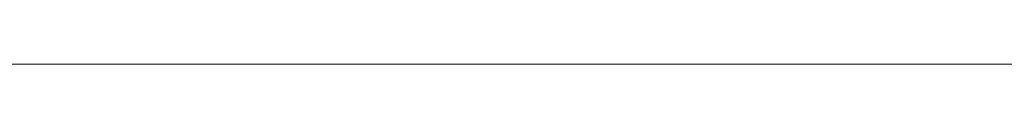
# Model space of a CAD drawing. Units: inches. Extents: x 459864 to 460310, y 324185 to 324787.
# Tile 89 of 112: x 460247.14006 to 460247.17582, y 324283.48323 to 324283.48324. Entities that reach past the tile are written whole.
import ezdxf

# ---------------------------------------------------------------- set-up
doc = ezdxf.new("R2010")
doc.units = ezdxf.units.IN
for name, color, linetype, lineweight in [('A-ANNO-DIMS', 2, 'Continuous', 18), ('L-HRDS', 9, 'Continuous', 18), ('L-SITE-PATT', 252, 'Continuous', 13)]:
    doc.layers.add(name, color=color, linetype=linetype, lineweight=lineweight)
doc.styles.get("Standard").update_dxf_attribs({"font": 'arial.ttf'})
doc.dimstyles.new('ISO-25', dxfattribs={"dimtxt": 6, "dimasz": 2.5, "dimexe": 1.25, "dimexo": 0.625, "dimtad": 1, "dimdec": 1, "dimlunit": 3, "dimtxsty": 'Standard', "dimcen": 2.5, "dimadec": 0, "dimazin": 0, "dimtfac": 1, "dimtdec": 1, "dimtmove": 0, "dimatfit": 3, "dimfxl": 1, "dimarcsym": 0})

# ---------------------------------------------------------------- blocks, each defined once
blk = doc.blocks.new('*D21')
at = {"layer": 'A-ANNO-DIMS', "color": 0, "lineweight": -2, "transparency": 16777216}
for p, q in [((460247.739927, 324715.483233), (460309.580369, 324715.483233)), ((460308.330369, 324712.983233), (460308.330369, 324285.983233)), ((460247.739927, 324283.483233), (460309.580369, 324283.483233))]:
    blk.add_line(p, q, dxfattribs=at)
at = {"layer": 'A-ANNO-DIMS', "color": 0, "transparency": 16777216}
for points in [[(460307.913702, 324712.983233), (460308.747035, 324712.983233), (460308.330369, 324715.483233)], [(460307.913702, 324285.983233), (460308.747035, 324285.983233), (460308.330369, 324283.483233)]]:
    blk.add_solid(points, dxfattribs=at)
at = {"layer": 'Defpoints', "color": 0, "transparency": 16777216}
for p in [(460247.114927, 324715.483233), (460247.114927, 324283.483233), (460308.330369, 324283.483233)]:
    blk.add_point(p, dxfattribs=at)
at = {"layer": 'A-ANNO-DIMS', "color": 0, "transparency": 16777216, "insert": (460304.639884, 324499.483233), "char_height": 6, "attachment_point": 5, "rotation": 90}
blk.add_mtext("36'", dxfattribs=at)

msp = doc.modelspace()

# ---------------------------------------------------------------- hatches: boundary and pattern name
at = {"layer": 'L-SITE-PATT'}
h = msp.add_hatch(dxfattribs=at)
h.set_pattern_fill('DOTS', color=256)
h.paths.add_polyline_path([(460269.803614, 324283.483233), (460247.114927, 324283.483233), (460121.929275, 324283.483233), (460121.929275, 324252.47302), (460117.429275, 324252.47302), (460110.123563, 324252.47302), (460110.123563, 324243.286537), (460080.829543, 324243.286537), (460080.829543, 324252.47302), (460061.114927, 324252.47302), (460061.114927, 324251.882422), (460077.9089, 324251.882422), (460077.9089, 324199.483233), (460080.829543, 324199.483233), (460080.829543, 324207.553216), (460110.123563, 324207.553216), (460110.123563, 324199.483233), (460110.813349, 324199.483233), (460262.114927, 324199.483233), (460269.803614, 324199.483233)], flags=17)
edge = h.paths.add_edge_path(flags=0)
edge.add_ellipse((460222.590295, 324263.813229), major_axis=(-8.485281, 8.485281), ratio=1, start_angle=405, end_angle=495, ccw=False)
edge.add_line((460214.820868, 324254.65989), (460214.831619, 324254.66592))
edge.add_ellipse((460222.590295, 324263.813229), major_axis=(-8.485281, 8.485281), ratio=1, start_angle=405, end_angle=495, ccw=False)
edge.add_line((460210.75891, 324261.780551), (460210.767583, 324261.786823))
edge.add_ellipse((460222.590295, 324263.813229), major_axis=(-8.485281, 8.485281), ratio=1, start_angle=405, end_angle=495, ccw=False)
edge.add_ellipse((460222.590295, 324263.813229), major_axis=(-8.485281, 8.485281), ratio=1, start_angle=392.754016, end_angle=405, ccw=False)
edge.add_ellipse((460222.590295, 324263.813229), major_axis=(-8.485281, 8.485281), ratio=1, start_angle=380.9347178, end_angle=392.754016, ccw=False)
edge.add_line((460211.337059, 324267.985029), (460211.340404, 324267.985029))
edge.add_ellipse((460222.590295, 324263.813229), major_axis=(-8.485281, 8.485281), ratio=1, start_angle=380.9347178, end_angle=392.754016, ccw=False)
edge.add_ellipse((460222.590295, 324263.813229), major_axis=(-8.485281, 8.485281), ratio=1, start_angle=347.9015209, end_angle=380.9347178, ccw=False)
edge.add_ellipse((460222.590295, 324263.813229), major_axis=(-8.485281, 8.485281), ratio=1, start_angle=327.0619241, end_angle=347.9015209, ccw=False)
edge.add_ellipse((460222.590295, 324263.813229), major_axis=(-8.485281, 8.485281), ratio=1, start_angle=278.3246418, end_angle=327.0619241, ccw=False)
edge.add_line((460225.158278, 324275.535991), (460225.157699, 324275.534637))
edge.add_ellipse((460222.590295, 324263.813229), major_axis=(-8.485281, 8.485281), ratio=1, start_angle=278.3246418, end_angle=327.0619241, ccw=False)
edge.add_ellipse((460222.590295, 324263.813229), major_axis=(-8.485281, 8.485281), ratio=1, start_angle=260.6435685, end_angle=278.3246418, ccw=False)
edge.add_ellipse((460222.590295, 324263.813229), major_axis=(-8.485281, 8.485281), ratio=1, start_angle=225, end_angle=260.6435685, ccw=False)
edge.add_line((460234.508791, 324265.242796), (460234.501456, 324265.239441))
edge.add_ellipse((460222.590295, 324263.813229), major_axis=(-8.485281, 8.485281), ratio=1, start_angle=225, end_angle=260.6435685, ccw=False)
edge.add_ellipse((460222.590295, 324263.813229), major_axis=(-8.485281, 8.485281), ratio=1, start_angle=495, end_angle=585, ccw=False)
edge.add_line((460234.436668, 324261.861215), (460234.423783, 324261.857822))
edge.add_ellipse((460222.590295, 324263.813229), major_axis=(-8.485281, 8.485281), ratio=1, start_angle=495, end_angle=585, ccw=False)
edge.add_line((460227.95013, 324253.067192), (460227.946414, 324253.083139))
edge.add_ellipse((460222.590295, 324263.813229), major_axis=(-8.485281, 8.485281), ratio=1, start_angle=495, end_angle=585, ccw=False)
edge.add_line((460226.222975, 324252.369267), (460226.21103, 324252.379551))
edge.add_ellipse((460222.590295, 324263.813229), major_axis=(-8.485281, 8.485281), ratio=1, start_angle=495, end_angle=585, ccw=False)
h.paths.add_polyline_path([(460219.651452, 324254.346654), (460218.461311, 324253.544985), (460218.275437, 324254.78932), (460219.642395, 324256.541765), (460219.62463, 324260.847564), (460216.110089, 324257.333022), (460214.349967, 324256.978066), (460215.416366, 324259.355678), (460212.523935, 324258.495823), (460213.137313, 324259.929797), (460218.507211, 324263.813229), (460222.590295, 324263.813229), (460222.590295, 324267.806698), (460218.175536, 324272.21231), (460219.025968, 324274.63898), (460222.590295, 324272.811129), (460222.590295, 324275.42332), (460223.057099, 324274.824931), (460222.67523, 324273.492211), (460225.911677, 324267.134611), (460219.62463, 324260.847564)], flags=0)
edge = h.paths.add_edge_path(flags=0)
edge.add_ellipse((460194.575758, 324264.046494), major_axis=(-8.485281, 8.485281), ratio=1, start_angle=495, end_angle=585, ccw=False)
edge.add_line((460199.935593, 324253.300458), (460199.931877, 324253.316405))
edge.add_ellipse((460194.575758, 324264.046494), major_axis=(-8.485281, 8.485281), ratio=1, start_angle=495, end_angle=585, ccw=False)
edge.add_line((460198.208438, 324252.602533), (460198.196493, 324252.612817))
edge.add_ellipse((460194.575758, 324264.046494), major_axis=(-8.485281, 8.485281), ratio=1, start_angle=495, end_angle=585, ccw=False)
edge.add_ellipse((460194.575758, 324264.046494), major_axis=(-8.485281, 8.485281), ratio=1, start_angle=405, end_angle=495, ccw=False)
edge.add_line((460186.806331, 324254.893156), (460186.817082, 324254.899186))
edge.add_ellipse((460194.575758, 324264.046494), major_axis=(-8.485281, 8.485281), ratio=1, start_angle=405, end_angle=495, ccw=False)
edge.add_line((460182.744373, 324262.013817), (460182.753046, 324262.020089))
edge.add_ellipse((460194.575758, 324264.046494), major_axis=(-8.485281, 8.485281), ratio=1, start_angle=405, end_angle=495, ccw=False)
edge.add_ellipse((460194.575758, 324264.046494), major_axis=(-8.485281, 8.485281), ratio=1, start_angle=392.754016, end_angle=405, ccw=False)
edge.add_ellipse((460194.575758, 324264.046494), major_axis=(-8.485281, 8.485281), ratio=1, start_angle=380.9347178, end_angle=392.754016, ccw=False)
edge.add_line((460183.322522, 324268.218294), (460183.325867, 324268.218294))
edge.add_ellipse((460194.575758, 324264.046494), major_axis=(-8.485281, 8.485281), ratio=1, start_angle=380.9347178, end_angle=392.754016, ccw=False)
edge.add_ellipse((460194.575758, 324264.046494), major_axis=(-8.485281, 8.485281), ratio=1, start_angle=347.9015209, end_angle=380.9347178, ccw=False)
edge.add_ellipse((460194.575758, 324264.046494), major_axis=(-8.485281, 8.485281), ratio=1, start_angle=327.0619241, end_angle=347.9015209, ccw=False)
edge.add_ellipse((460194.575758, 324264.046494), major_axis=(-8.485281, 8.485281), ratio=1, start_angle=278.3246418, end_angle=327.0619241, ccw=False)
edge.add_line((460197.143741, 324275.769257), (460197.143162, 324275.767903))
edge.add_ellipse((460194.575758, 324264.046494), major_axis=(-8.485281, 8.485281), ratio=1, start_angle=278.3246418, end_angle=327.0619241, ccw=False)
edge.add_ellipse((460194.575758, 324264.046494), major_axis=(-8.485281, 8.485281), ratio=1, start_angle=260.6435685, end_angle=278.3246418, ccw=False)
edge.add_ellipse((460194.575758, 324264.046494), major_axis=(-8.485281, 8.485281), ratio=1, start_angle=225, end_angle=260.6435685, ccw=False)
edge.add_line((460206.494254, 324265.476062), (460206.486919, 324265.472707))
edge.add_ellipse((460194.575758, 324264.046494), major_axis=(-8.485281, 8.485281), ratio=1, start_angle=225, end_angle=260.6435685, ccw=False)
edge.add_ellipse((460194.575758, 324264.046494), major_axis=(-8.485281, 8.485281), ratio=1, start_angle=495, end_angle=585, ccw=False)
edge.add_line((460206.422132, 324262.094481), (460206.409246, 324262.091088))
h.paths.add_polyline_path([(460191.610093, 324261.08083), (460191.636915, 324254.57992), (460190.446774, 324253.778251), (460190.2609, 324255.022585), (460191.627858, 324256.775031), (460191.610093, 324261.08083), (460188.095552, 324257.566288), (460186.33543, 324257.211332), (460187.40183, 324259.588944), (460184.509398, 324258.729088), (460185.122776, 324260.163063), (460190.492675, 324264.046494), (460194.575758, 324264.046494), (460194.575758, 324268.039963), (460190.160999, 324272.445576), (460191.011431, 324274.872246), (460194.575758, 324273.044395), (460194.575758, 324275.656585), (460195.042562, 324275.058197), (460194.660693, 324273.725477), (460197.897141, 324267.367877)], flags=0)
edge = h.paths.add_edge_path(flags=0)
edge.add_ellipse((460252.911961, 324263.577616), major_axis=(-8.485281, 8.485281), ratio=1, start_angle=405, end_angle=495, ccw=False)
edge.add_line((460241.080576, 324261.544938), (460241.089249, 324261.55121))
edge.add_ellipse((460252.911961, 324263.577616), major_axis=(-8.485281, 8.485281), ratio=1, start_angle=405, end_angle=495, ccw=False)
edge.add_ellipse((460252.911961, 324263.577616), major_axis=(-8.485281, 8.485281), ratio=1, start_angle=392.754016, end_angle=405, ccw=False)
edge.add_ellipse((460252.911961, 324263.577616), major_axis=(-8.485281, 8.485281), ratio=1, start_angle=380.9347178, end_angle=392.754016, ccw=False)
edge.add_line((460241.658725, 324267.749416), (460241.66207, 324267.749416))
edge.add_ellipse((460252.911961, 324263.577616), major_axis=(-8.485281, 8.485281), ratio=1, start_angle=380.9347178, end_angle=392.754016, ccw=False)
edge.add_ellipse((460252.911961, 324263.577616), major_axis=(-8.485281, 8.485281), ratio=1, start_angle=347.9015209, end_angle=380.9347178, ccw=False)
edge.add_ellipse((460252.911961, 324263.577616), major_axis=(-8.485281, 8.485281), ratio=1, start_angle=327.0619241, end_angle=347.9015209, ccw=False)
edge.add_ellipse((460252.911961, 324263.577616), major_axis=(-8.485281, 8.485281), ratio=1, start_angle=278.3246418, end_angle=327.0619241, ccw=False)
edge.add_line((460255.479944, 324275.300378), (460255.479365, 324275.299024))
edge.add_ellipse((460252.911961, 324263.577616), major_axis=(-8.485281, 8.485281), ratio=1, start_angle=278.3246418, end_angle=327.0619241, ccw=False)
edge.add_ellipse((460252.911961, 324263.577616), major_axis=(-8.485281, 8.485281), ratio=1, start_angle=260.6435685, end_angle=278.3246418, ccw=False)
edge.add_ellipse((460252.911961, 324263.577616), major_axis=(-8.485281, 8.485281), ratio=1, start_angle=225, end_angle=260.6435685, ccw=False)
edge.add_line((460264.830457, 324265.007183), (460264.823122, 324265.003828))
edge.add_ellipse((460252.911961, 324263.577616), major_axis=(-8.485281, 8.485281), ratio=1, start_angle=225, end_angle=260.6435685, ccw=False)
edge.add_ellipse((460252.911961, 324263.577616), major_axis=(-8.485281, 8.485281), ratio=1, start_angle=495, end_angle=585, ccw=False)
edge.add_line((460264.758335, 324261.625602), (460264.745449, 324261.622209))
edge.add_ellipse((460252.911961, 324263.577616), major_axis=(-8.485281, 8.485281), ratio=1, start_angle=495, end_angle=585, ccw=False)
edge.add_line((460258.271796, 324252.831579), (460258.268081, 324252.847526))
edge.add_ellipse((460252.911961, 324263.577616), major_axis=(-8.485281, 8.485281), ratio=1, start_angle=495, end_angle=585, ccw=False)
edge.add_line((460256.544641, 324252.133654), (460256.532696, 324252.143938))
edge.add_ellipse((460252.911961, 324263.577616), major_axis=(-8.485281, 8.485281), ratio=1, start_angle=495, end_angle=585, ccw=False)
edge.add_ellipse((460252.911961, 324263.577616), major_axis=(-8.485281, 8.485281), ratio=1, start_angle=405, end_angle=495, ccw=False)
edge.add_line((460245.142534, 324254.424277), (460245.153285, 324254.430307))
h.paths.add_polyline_path([(460244.671633, 324256.742453), (460245.738033, 324259.120065), (460242.845601, 324258.26021), (460243.458979, 324259.694184), (460248.828878, 324263.577616), (460252.911961, 324263.577616), (460252.911961, 324267.571085), (460248.497202, 324271.976697), (460249.347634, 324274.403367), (460252.911961, 324272.575516), (460252.911961, 324275.187707), (460253.378765, 324274.589318), (460252.996897, 324273.256598), (460256.233344, 324266.898998), (460249.946296, 324260.611951), (460249.973118, 324254.111041), (460248.782977, 324253.309372), (460248.597103, 324254.553707), (460249.964061, 324256.306152), (460249.946296, 324260.611951), (460246.431755, 324257.097409)], flags=0)
edge = h.paths.add_edge_path(flags=0)
edge.add_ellipse((460167.43869, 324262.832792), major_axis=(-8.485281, 8.485281), ratio=1, start_angle=495, end_angle=585, ccw=False)
edge.add_line((460172.798524, 324252.086755), (460172.794809, 324252.102702))
edge.add_ellipse((460167.43869, 324262.832792), major_axis=(-8.485281, 8.485281), ratio=1, start_angle=495, end_angle=585, ccw=False)
edge.add_line((460171.07137, 324251.38883), (460171.059425, 324251.399114))
edge.add_ellipse((460167.43869, 324262.832792), major_axis=(-8.485281, 8.485281), ratio=1, start_angle=495, end_angle=585, ccw=False)
edge.add_ellipse((460167.43869, 324262.832792), major_axis=(-8.485281, 8.485281), ratio=1, start_angle=405, end_angle=495, ccw=False)
edge.add_line((460159.669262, 324253.679453), (460159.680013, 324253.685483))
edge.add_ellipse((460167.43869, 324262.832792), major_axis=(-8.485281, 8.485281), ratio=1, start_angle=405, end_angle=495, ccw=False)
edge.add_line((460155.607304, 324260.800114), (460155.615977, 324260.806386))
edge.add_ellipse((460167.43869, 324262.832792), major_axis=(-8.485281, 8.485281), ratio=1, start_angle=405, end_angle=495, ccw=False)
edge.add_ellipse((460167.43869, 324262.832792), major_axis=(-8.485281, 8.485281), ratio=1, start_angle=392.754016, end_angle=405, ccw=False)
edge.add_ellipse((460167.43869, 324262.832792), major_axis=(-8.485281, 8.485281), ratio=1, start_angle=380.9347178, end_angle=392.754016, ccw=False)
edge.add_line((460156.185453, 324267.004592), (460156.188798, 324267.004592))
edge.add_ellipse((460167.43869, 324262.832792), major_axis=(-8.485281, 8.485281), ratio=1, start_angle=380.9347178, end_angle=392.754016, ccw=False)
edge.add_ellipse((460167.43869, 324262.832792), major_axis=(-8.485281, 8.485281), ratio=1, start_angle=347.9015209, end_angle=380.9347178, ccw=False)
edge.add_ellipse((460167.43869, 324262.832792), major_axis=(-8.485281, 8.485281), ratio=1, start_angle=327.0619241, end_angle=347.9015209, ccw=False)
edge.add_ellipse((460167.43869, 324262.832792), major_axis=(-8.485281, 8.485281), ratio=1, start_angle=278.3246418, end_angle=327.0619241, ccw=False)
edge.add_line((460170.006672, 324274.555554), (460170.006093, 324274.5542))
edge.add_ellipse((460167.43869, 324262.832792), major_axis=(-8.485281, 8.485281), ratio=1, start_angle=278.3246418, end_angle=327.0619241, ccw=False)
edge.add_ellipse((460167.43869, 324262.832792), major_axis=(-8.485281, 8.485281), ratio=1, start_angle=260.6435685, end_angle=278.3246418, ccw=False)
edge.add_ellipse((460167.43869, 324262.832792), major_axis=(-8.485281, 8.485281), ratio=1, start_angle=225, end_angle=260.6435685, ccw=False)
edge.add_line((460179.357186, 324264.262359), (460179.349851, 324264.259004))
edge.add_ellipse((460167.43869, 324262.832792), major_axis=(-8.485281, 8.485281), ratio=1, start_angle=225, end_angle=260.6435685, ccw=False)
edge.add_ellipse((460167.43869, 324262.832792), major_axis=(-8.485281, 8.485281), ratio=1, start_angle=495, end_angle=585, ccw=False)
edge.add_line((460179.285063, 324260.880778), (460179.272177, 324260.877385))
h.paths.add_polyline_path([(460164.473025, 324259.867127), (460164.499846, 324253.366217), (460163.309706, 324252.564548), (460163.123831, 324253.808883), (460164.49079, 324255.561328), (460164.473025, 324259.867127), (460160.958483, 324256.352585), (460159.198362, 324255.997629), (460160.264761, 324258.375241), (460157.372329, 324257.515386), (460157.985707, 324258.94936), (460163.355606, 324262.832792), (460167.43869, 324262.832792), (460167.43869, 324266.826261), (460163.02393, 324271.231873), (460163.874362, 324273.658543), (460167.43869, 324271.830692), (460167.43869, 324274.442883), (460167.905493, 324273.844494), (460167.523625, 324272.511774), (460170.760072, 324266.154174)], flags=0)
edge = h.paths.add_edge_path(flags=0)
edge.add_ellipse((460140.758089, 324262.369585), major_axis=(-8.485281, 8.485281), ratio=1, start_angle=495, end_angle=585, ccw=False)
edge.add_line((460146.117923, 324251.623548), (460146.114208, 324251.639495))
edge.add_ellipse((460140.758089, 324262.369585), major_axis=(-8.485281, 8.485281), ratio=1, start_angle=495, end_angle=585, ccw=False)
edge.add_line((460144.390769, 324250.925623), (460144.378824, 324250.935907))
edge.add_ellipse((460140.758089, 324262.369585), major_axis=(-8.485281, 8.485281), ratio=1, start_angle=495, end_angle=585, ccw=False)
edge.add_ellipse((460140.758089, 324262.369585), major_axis=(-8.485281, 8.485281), ratio=1, start_angle=405, end_angle=495, ccw=False)
edge.add_line((460132.988661, 324253.216246), (460132.999412, 324253.222276))
edge.add_ellipse((460140.758089, 324262.369585), major_axis=(-8.485281, 8.485281), ratio=1, start_angle=405, end_angle=495, ccw=False)
edge.add_line((460128.926703, 324260.336907), (460128.935376, 324260.343179))
edge.add_ellipse((460140.758089, 324262.369585), major_axis=(-8.485281, 8.485281), ratio=1, start_angle=405, end_angle=495, ccw=False)
edge.add_ellipse((460140.758089, 324262.369585), major_axis=(-8.485281, 8.485281), ratio=1, start_angle=392.754016, end_angle=405, ccw=False)
edge.add_ellipse((460140.758089, 324262.369585), major_axis=(-8.485281, 8.485281), ratio=1, start_angle=380.9347178, end_angle=392.754016, ccw=False)
edge.add_line((460129.504852, 324266.541385), (460129.508197, 324266.541385))
edge.add_ellipse((460140.758089, 324262.369585), major_axis=(-8.485281, 8.485281), ratio=1, start_angle=380.9347178, end_angle=392.754016, ccw=False)
edge.add_ellipse((460140.758089, 324262.369585), major_axis=(-8.485281, 8.485281), ratio=1, start_angle=347.9015209, end_angle=380.9347178, ccw=False)
edge.add_ellipse((460140.758089, 324262.369585), major_axis=(-8.485281, 8.485281), ratio=1, start_angle=327.0619241, end_angle=347.9015209, ccw=False)
edge.add_ellipse((460140.758089, 324262.369585), major_axis=(-8.485281, 8.485281), ratio=1, start_angle=278.3246418, end_angle=327.0619241, ccw=False)
edge.add_line((460143.326071, 324274.092347), (460143.325492, 324274.090993))
edge.add_ellipse((460140.758089, 324262.369585), major_axis=(-8.485281, 8.485281), ratio=1, start_angle=278.3246418, end_angle=327.0619241, ccw=False)
edge.add_ellipse((460140.758089, 324262.369585), major_axis=(-8.485281, 8.485281), ratio=1, start_angle=260.6435685, end_angle=278.3246418, ccw=False)
edge.add_ellipse((460140.758089, 324262.369585), major_axis=(-8.485281, 8.485281), ratio=1, start_angle=225, end_angle=260.6435685, ccw=False)
edge.add_line((460152.676585, 324263.799152), (460152.66925, 324263.795797))
edge.add_ellipse((460140.758089, 324262.369585), major_axis=(-8.485281, 8.485281), ratio=1, start_angle=225, end_angle=260.6435685, ccw=False)
edge.add_ellipse((460140.758089, 324262.369585), major_axis=(-8.485281, 8.485281), ratio=1, start_angle=495, end_angle=585, ccw=False)
edge.add_line((460152.604462, 324260.417571), (460152.591576, 324260.414178))
h.paths.add_polyline_path([(460137.792424, 324259.40392), (460137.819245, 324252.90301), (460136.629105, 324252.101341), (460136.44323, 324253.345676), (460137.810189, 324255.098121), (460137.792424, 324259.40392), (460134.277882, 324255.889378), (460132.517761, 324255.534422), (460133.58416, 324257.912034), (460130.691728, 324257.052179), (460131.305106, 324258.486153), (460136.675005, 324262.369585), (460140.758089, 324262.369585), (460140.758089, 324266.363054), (460136.343329, 324270.768666), (460137.193761, 324273.195336), (460140.758089, 324271.367485), (460140.758089, 324273.979676), (460141.224892, 324273.381287), (460140.843024, 324272.048567), (460144.079471, 324265.690967)], flags=0)
h.paths.add_polyline_path([(460110.123563, 324227.413868), (460080.829543, 324227.413868), (460080.829543, 324235.483851), (460110.123563, 324235.483851)], flags=16)
h.paths.add_polyline_path([(460110.123563, 324220.796634), (460110.123563, 324212.726651), (460080.829543, 324212.726651), (460080.829543, 324220.796634)], flags=16)
h.paths.add_polyline_path([(460269.803614, 324283.483233), (460247.114927, 324283.483233), (460121.929275, 324283.483233), (460121.929275, 324252.47302), (460117.429275, 324252.47302), (460110.123563, 324252.47302), (460110.123563, 324243.286537), (460080.829543, 324243.286537), (460080.829543, 324252.47302), (460061.114927, 324252.47302), (460061.114927, 324251.882422), (460077.9089, 324251.882422), (460077.9089, 324199.483233), (460080.829543, 324199.483233), (460080.829543, 324207.553216), (460110.123563, 324207.553216), (460110.123563, 324199.483233), (460262.114927, 324199.483233), (460269.803614, 324199.483233)], flags=17)
h.paths.add_polyline_path([(460219.651452, 324254.346654), (460218.461311, 324253.544985), (460218.275437, 324254.78932), (460219.642395, 324256.541765), (460219.62463, 324260.847564), (460216.110089, 324257.333022), (460214.349967, 324256.978066), (460215.416366, 324259.355678), (460212.523935, 324258.495823), (460213.137313, 324259.929797), (460218.507211, 324263.813229), (460222.590295, 324263.813229), (460220.180486, 324266.223037), (460215.460959, 324265.307646), (460211.834533, 324266.136551), (460216.246619, 324267.985029), (460218.418495, 324267.985029), (460222.590295, 324263.813229), (460222.590295, 324267.806698), (460218.175536, 324272.21231), (460219.025968, 324274.63898), (460222.590295, 324272.811129), (460222.590295, 324275.42332), (460223.057099, 324274.824931), (460222.67523, 324273.492211), (460225.911677, 324267.134611), (460222.590295, 324263.813229), (460231.382871, 324263.813229), (460228.484718, 324262.487825), (460224.425208, 324261.978316), (460228.679899, 324257.723625), (460228.965835, 324254.791014), (460227.141768, 324256.536632), (460227.542067, 324254.818575), (460227.333342, 324253.614466), (460222.590295, 324259.984626), (460222.590295, 324255.496666), (460221.377409, 324256.540849), (460220.575794, 324261.798728), (460219.62463, 324260.847564)], flags=0)
h.paths.add_polyline_path([(460199.127231, 324256.769898), (460199.52753, 324255.051841), (460199.318805, 324253.847732), (460194.575758, 324260.217892), (460194.575758, 324255.729932), (460193.362872, 324256.774115), (460192.561257, 324262.031993), (460191.610093, 324261.08083), (460191.636915, 324254.57992), (460190.446774, 324253.778251), (460190.2609, 324255.022585), (460191.627858, 324256.775031), (460191.610093, 324261.08083), (460188.095552, 324257.566288), (460186.33543, 324257.211332), (460187.40183, 324259.588944), (460184.509398, 324258.729088), (460185.122776, 324260.163063), (460190.492675, 324264.046494), (460194.575758, 324264.046494), (460192.16595, 324266.456303), (460187.446422, 324265.540912), (460183.819996, 324266.369816), (460188.232082, 324268.218294), (460190.403958, 324268.218294), (460194.575758, 324264.046494), (460194.575758, 324268.039963), (460190.160999, 324272.445576), (460191.011431, 324274.872246), (460194.575758, 324273.044395), (460194.575758, 324275.656585), (460195.042562, 324275.058197), (460194.660693, 324273.725477), (460197.897141, 324267.367877), (460194.575758, 324264.046494), (460203.368334, 324264.046494), (460200.470181, 324262.721091), (460196.410671, 324262.211582), (460200.665362, 324257.956891), (460200.951298, 324255.02428)], flags=0)
h.paths.add_polyline_path([(460244.671633, 324256.742453), (460245.738033, 324259.120065), (460242.845601, 324258.26021), (460243.458979, 324259.694184), (460248.828878, 324263.577616), (460252.911961, 324263.577616), (460250.502153, 324265.987424), (460245.782625, 324265.072033), (460242.156199, 324265.900938), (460246.568285, 324267.749416), (460248.740161, 324267.749416), (460252.911961, 324263.577616), (460252.911961, 324267.571085), (460248.497202, 324271.976697), (460249.347634, 324274.403367), (460252.911961, 324272.575516), (460252.911961, 324275.187707), (460253.378765, 324274.589318), (460252.996897, 324273.256598), (460256.233344, 324266.898998), (460252.911961, 324263.577616), (460261.704537, 324263.577616), (460258.806384, 324262.252212), (460254.746874, 324261.742703), (460259.001565, 324257.488012), (460259.287501, 324254.555401), (460257.463434, 324256.301019), (460257.863733, 324254.582962), (460257.655008, 324253.378853), (460252.911961, 324259.749013), (460252.911961, 324255.261053), (460251.699075, 324256.305236), (460250.89746, 324261.563115), (460249.946296, 324260.611951), (460249.973118, 324254.111041), (460248.782977, 324253.309372), (460248.597103, 324254.553707), (460249.964061, 324256.306152), (460249.946296, 324260.611951), (460246.431755, 324257.097409)], flags=0)
h.paths.add_polyline_path([(460173.528293, 324256.743188), (460173.81423, 324253.810577), (460171.990163, 324255.556195), (460172.390461, 324253.838138), (460172.181736, 324252.634029), (460167.43869, 324259.004189), (460167.43869, 324254.516229), (460166.225803, 324255.560412), (460165.424189, 324260.818291), (460164.473025, 324259.867127), (460164.499846, 324253.366217), (460163.309706, 324252.564548), (460163.123831, 324253.808883), (460164.49079, 324255.561328), (460164.473025, 324259.867127), (460160.958483, 324256.352585), (460159.198362, 324255.997629), (460160.264761, 324258.375241), (460157.372329, 324257.515386), (460157.985707, 324258.94936), (460163.355606, 324262.832792), (460167.43869, 324262.832792), (460165.028881, 324265.2426), (460160.309353, 324264.327209), (460156.682927, 324265.156114), (460161.095013, 324267.004592), (460163.26689, 324267.004592), (460167.43869, 324262.832792), (460167.43869, 324266.826261), (460163.02393, 324271.231873), (460163.874362, 324273.658543), (460167.43869, 324271.830692), (460167.43869, 324274.442883), (460167.905493, 324273.844494), (460167.523625, 324272.511774), (460170.760072, 324266.154174), (460167.43869, 324262.832792), (460176.231266, 324262.832792), (460173.333113, 324261.507388), (460169.273603, 324260.997879)], flags=0)
h.paths.add_polyline_path([(460146.847692, 324256.279981), (460147.133629, 324253.34737), (460145.309562, 324255.092988), (460145.70986, 324253.374931), (460145.501135, 324252.170822), (460140.758089, 324258.540983), (460140.758089, 324254.053022), (460139.545202, 324255.097205), (460138.743588, 324260.355084), (460137.792424, 324259.40392), (460137.819245, 324252.90301), (460136.629105, 324252.101341), (460136.44323, 324253.345676), (460137.810189, 324255.098121), (460137.792424, 324259.40392), (460134.277882, 324255.889378), (460132.517761, 324255.534422), (460133.58416, 324257.912034), (460130.691728, 324257.052179), (460131.305106, 324258.486153), (460136.675005, 324262.369585), (460140.758089, 324262.369585), (460138.34828, 324264.779393), (460133.628752, 324263.864002), (460130.002326, 324264.692907), (460134.414412, 324266.541385), (460136.586289, 324266.541385), (460140.758089, 324262.369585), (460140.758089, 324266.363054), (460136.343329, 324270.768666), (460137.193761, 324273.195336), (460140.758089, 324271.367485), (460140.758089, 324273.979676), (460141.224892, 324273.381287), (460140.843024, 324272.048567), (460144.079471, 324265.690967), (460140.758089, 324262.369585), (460149.550664, 324262.369585), (460146.652512, 324261.044182), (460142.593002, 324260.534672)], flags=0)
edge = h.paths.add_edge_path()
edge.add_line((460269.803614, 324272.549054), (460260.881484, 324272.549054))
edge.add_ellipse((460252.911961, 324263.577616), major_axis=(-8.485281, 8.485281), ratio=1, start_angle=260.6435685, end_angle=273.3846244, ccw=False)
edge.add_line((460262.282614, 324271.092108), (460262.260554, 324271.09106))
edge.add_ellipse((460252.911961, 324263.577616), major_axis=(-8.485281, 8.485281), ratio=1, start_angle=260.6435685, end_angle=273.3846244, ccw=False)
edge.add_ellipse((460252.911961, 324263.577616), major_axis=(-8.485281, 8.485281), ratio=1, start_angle=225, end_angle=260.6435685, ccw=False)
edge.add_line((460263.608568, 324269.063294), (460263.571652, 324269.058283))
edge.add_ellipse((460252.911961, 324263.577616), major_axis=(-8.485281, 8.485281), ratio=1, start_angle=225, end_angle=260.6435685, ccw=False)
edge.add_line((460264.615462, 324266.30554), (460264.585358, 324266.305196))
edge.add_ellipse((460252.911961, 324263.577616), major_axis=(-8.485281, 8.485281), ratio=1, start_angle=225, end_angle=260.6435685, ccw=False)
edge.add_line((460264.830457, 324265.007183), (460264.823122, 324265.003828))
edge.add_ellipse((460252.911961, 324263.577616), major_axis=(-8.485281, 8.485281), ratio=1, start_angle=225, end_angle=260.6435685, ccw=False)
edge.add_ellipse((460252.911961, 324263.577616), major_axis=(-8.485281, 8.485281), ratio=1, start_angle=495, end_angle=585, ccw=False)
edge.add_line((460264.758335, 324261.625602), (460264.745449, 324261.622209))
edge.add_ellipse((460252.911961, 324263.577616), major_axis=(-8.485281, 8.485281), ratio=1, start_angle=495, end_angle=585, ccw=False)
edge.add_line((460263.442202, 324257.739018), (460263.389259, 324257.779239))
edge.add_ellipse((460252.911961, 324263.577616), major_axis=(-8.485281, 8.485281), ratio=1, start_angle=495, end_angle=585, ccw=False)
edge.add_line((460258.128071, 324252.743505), (460258.101878, 324252.778683))
edge.add_ellipse((460252.911961, 324263.577616), major_axis=(-8.485281, 8.485281), ratio=1, start_angle=495, end_angle=585, ccw=False)
edge.add_line((460256.544641, 324252.133654), (460256.532696, 324252.143938))
edge.add_ellipse((460252.911961, 324263.577616), major_axis=(-8.485281, 8.485281), ratio=1, start_angle=495, end_angle=585, ccw=False)
edge.add_ellipse((460252.911961, 324263.577616), major_axis=(-8.485281, 8.485281), ratio=1, start_angle=405, end_angle=495, ccw=False)
edge.add_line((460250.593989, 324251.780412), (460250.604653, 324251.819817))
edge.add_ellipse((460252.911961, 324263.577616), major_axis=(-8.485281, 8.485281), ratio=1, start_angle=405, end_angle=495, ccw=False)
edge.add_line((460245.142534, 324254.424277), (460245.153285, 324254.430307))
edge.add_ellipse((460252.911961, 324263.577616), major_axis=(-8.485281, 8.485281), ratio=1, start_angle=405, end_angle=495, ccw=False)
edge.add_line((460243.524588, 324256.059004), (460243.560343, 324256.091361))
edge.add_ellipse((460252.911961, 324263.577616), major_axis=(-8.485281, 8.485281), ratio=1, start_angle=405, end_angle=495, ccw=False)
edge.add_line((460241.440103, 324259.892726), (460241.522441, 324259.895877))
edge.add_ellipse((460252.911961, 324263.577616), major_axis=(-8.485281, 8.485281), ratio=1, start_angle=405, end_angle=495, ccw=False)
edge.add_line((460241.080576, 324261.544938), (460241.089249, 324261.55121))
edge.add_ellipse((460252.911961, 324263.577616), major_axis=(-8.485281, 8.485281), ratio=1, start_angle=405, end_angle=495, ccw=False)
edge.add_ellipse((460252.911961, 324263.577616), major_axis=(-8.485281, 8.485281), ratio=1, start_angle=392.754016, end_angle=405, ccw=False)
edge.add_line((460241.050299, 324265.437612), (460241.062566, 324265.442751))
edge.add_ellipse((460252.911961, 324263.577616), major_axis=(-8.485281, 8.485281), ratio=1, start_angle=392.754016, end_angle=405, ccw=False)
edge.add_ellipse((460252.911961, 324263.577616), major_axis=(-8.485281, 8.485281), ratio=1, start_angle=380.9347178, end_angle=392.754016, ccw=False)
edge.add_line((460241.451888, 324267.176391), (460241.469044, 324267.170988))
edge.add_ellipse((460252.911961, 324263.577616), major_axis=(-8.485281, 8.485281), ratio=1, start_angle=380.9347178, end_angle=392.754016, ccw=False)
edge.add_line((460241.658725, 324267.749416), (460241.66207, 324267.749416))
edge.add_ellipse((460252.911961, 324263.577616), major_axis=(-8.485281, 8.485281), ratio=1, start_angle=380.9347178, end_angle=392.754016, ccw=False)
edge.add_ellipse((460252.911961, 324263.577616), major_axis=(-8.485281, 8.485281), ratio=1, start_angle=356.6153756, end_angle=380.9347178, ccw=False)
edge.add_line((460244.880293, 324272.487651), (460244.712651, 324272.549054))
edge.add_line((460244.712651, 324272.549054), (460230.817406, 324272.549054))
edge.add_ellipse((460222.590295, 324263.813229), major_axis=(-8.485281, 8.485281), ratio=1, start_angle=260.6435685, end_angle=271.7177746, ccw=False)
edge.add_ellipse((460222.590295, 324263.813229), major_axis=(-8.485281, 8.485281), ratio=1, start_angle=225, end_angle=260.6435685, ccw=False)
edge.add_line((460233.286902, 324269.298907), (460233.249986, 324269.293896))
edge.add_ellipse((460222.590295, 324263.813229), major_axis=(-8.485281, 8.485281), ratio=1, start_angle=225, end_angle=260.6435685, ccw=False)
edge.add_line((460234.293796, 324266.541153), (460234.263692, 324266.540809))
edge.add_ellipse((460222.590295, 324263.813229), major_axis=(-8.485281, 8.485281), ratio=1, start_angle=225, end_angle=260.6435685, ccw=False)
edge.add_line((460234.508791, 324265.242796), (460234.501456, 324265.239441))
edge.add_ellipse((460222.590295, 324263.813229), major_axis=(-8.485281, 8.485281), ratio=1, start_angle=225, end_angle=260.6435685, ccw=False)
edge.add_ellipse((460222.590295, 324263.813229), major_axis=(-8.485281, 8.485281), ratio=1, start_angle=495, end_angle=585, ccw=False)
edge.add_line((460234.436668, 324261.861215), (460234.423783, 324261.857822))
edge.add_ellipse((460222.590295, 324263.813229), major_axis=(-8.485281, 8.485281), ratio=1, start_angle=495, end_angle=585, ccw=False)
edge.add_line((460233.120535, 324257.974631), (460233.067593, 324258.014852))
edge.add_ellipse((460222.590295, 324263.813229), major_axis=(-8.485281, 8.485281), ratio=1, start_angle=495, end_angle=585, ccw=False)
edge.add_line((460227.806405, 324252.979118), (460227.780212, 324253.014296))
edge.add_ellipse((460222.590295, 324263.813229), major_axis=(-8.485281, 8.485281), ratio=1, start_angle=495, end_angle=585, ccw=False)
edge.add_line((460226.222975, 324252.369267), (460226.21103, 324252.379551))
edge.add_ellipse((460222.590295, 324263.813229), major_axis=(-8.485281, 8.485281), ratio=1, start_angle=495, end_angle=585, ccw=False)
edge.add_ellipse((460222.590295, 324263.813229), major_axis=(-8.485281, 8.485281), ratio=1, start_angle=405, end_angle=495, ccw=False)
edge.add_line((460220.272323, 324252.016025), (460220.282987, 324252.05543))
edge.add_ellipse((460222.590295, 324263.813229), major_axis=(-8.485281, 8.485281), ratio=1, start_angle=405, end_angle=495, ccw=False)
edge.add_line((460214.820868, 324254.65989), (460214.831619, 324254.66592))
edge.add_ellipse((460222.590295, 324263.813229), major_axis=(-8.485281, 8.485281), ratio=1, start_angle=405, end_angle=495, ccw=False)
edge.add_line((460213.202922, 324256.294617), (460213.238677, 324256.326974))
edge.add_ellipse((460222.590295, 324263.813229), major_axis=(-8.485281, 8.485281), ratio=1, start_angle=405, end_angle=495, ccw=False)
edge.add_line((460211.118437, 324260.128339), (460211.200774, 324260.13149))
edge.add_ellipse((460222.590295, 324263.813229), major_axis=(-8.485281, 8.485281), ratio=1, start_angle=405, end_angle=495, ccw=False)
edge.add_line((460210.75891, 324261.780551), (460210.767583, 324261.786823))
edge.add_ellipse((460222.590295, 324263.813229), major_axis=(-8.485281, 8.485281), ratio=1, start_angle=405, end_angle=495, ccw=False)
edge.add_ellipse((460222.590295, 324263.813229), major_axis=(-8.485281, 8.485281), ratio=1, start_angle=392.754016, end_angle=405, ccw=False)
edge.add_line((460210.728633, 324265.673225), (460210.7409, 324265.678364))
edge.add_ellipse((460222.590295, 324263.813229), major_axis=(-8.485281, 8.485281), ratio=1, start_angle=392.754016, end_angle=405, ccw=False)
edge.add_ellipse((460222.590295, 324263.813229), major_axis=(-8.485281, 8.485281), ratio=1, start_angle=380.9347178, end_angle=392.754016, ccw=False)
edge.add_line((460211.130222, 324267.412004), (460211.147378, 324267.406601))
edge.add_ellipse((460222.590295, 324263.813229), major_axis=(-8.485281, 8.485281), ratio=1, start_angle=380.9347178, end_angle=392.754016, ccw=False)
edge.add_line((460211.337059, 324267.985029), (460211.340404, 324267.985029))
edge.add_ellipse((460222.590295, 324263.813229), major_axis=(-8.485281, 8.485281), ratio=1, start_angle=380.9347178, end_angle=392.754016, ccw=False)
edge.add_ellipse((460222.590295, 324263.813229), major_axis=(-8.485281, 8.485281), ratio=1, start_angle=358.2822254, end_angle=380.9347178, ccw=False)
edge.add_line((460213.704522, 324271.901826), (460213.709044, 324271.868974))
edge.add_ellipse((460222.590295, 324263.813229), major_axis=(-8.485281, 8.485281), ratio=1, start_angle=358.2822254, end_angle=380.9347178, ccw=False)
edge.add_line((460214.363185, 324272.549054), (460203.078318, 324272.549054))
edge.add_line((460203.078318, 324272.549054), (460203.060342, 324272.531078))
edge.add_ellipse((460194.575758, 324264.046494), major_axis=(-8.485281, 8.485281), ratio=1, start_angle=260.6435685, end_angle=270.11679, ccw=False)
edge.add_line((460203.956591, 324271.56147), (460203.920907, 324271.559776))
edge.add_ellipse((460194.575758, 324264.046494), major_axis=(-8.485281, 8.485281), ratio=1, start_angle=260.6435685, end_angle=270.11679, ccw=False)
edge.add_ellipse((460194.575758, 324264.046494), major_axis=(-8.485281, 8.485281), ratio=1, start_angle=225, end_angle=260.6435685, ccw=False)
edge.add_line((460205.272365, 324269.532172), (460205.235449, 324269.527161))
edge.add_ellipse((460194.575758, 324264.046494), major_axis=(-8.485281, 8.485281), ratio=1, start_angle=225, end_angle=260.6435685, ccw=False)
edge.add_line((460206.279259, 324266.774419), (460206.249155, 324266.774075))
edge.add_ellipse((460194.575758, 324264.046494), major_axis=(-8.485281, 8.485281), ratio=1, start_angle=225, end_angle=260.6435685, ccw=False)
edge.add_line((460206.494254, 324265.476062), (460206.486919, 324265.472707))
edge.add_ellipse((460194.575758, 324264.046494), major_axis=(-8.485281, 8.485281), ratio=1, start_angle=225, end_angle=260.6435685, ccw=False)
edge.add_ellipse((460194.575758, 324264.046494), major_axis=(-8.485281, 8.485281), ratio=1, start_angle=495, end_angle=585, ccw=False)
edge.add_line((460206.422132, 324262.094481), (460206.409246, 324262.091088))
edge.add_ellipse((460194.575758, 324264.046494), major_axis=(-8.485281, 8.485281), ratio=1, start_angle=495, end_angle=585, ccw=False)
edge.add_line((460205.105999, 324258.207897), (460205.053056, 324258.248118))
edge.add_ellipse((460194.575758, 324264.046494), major_axis=(-8.485281, 8.485281), ratio=1, start_angle=495, end_angle=585, ccw=False)
edge.add_line((460199.791868, 324253.212383), (460199.765675, 324253.247562))
edge.add_ellipse((460194.575758, 324264.046494), major_axis=(-8.485281, 8.485281), ratio=1, start_angle=495, end_angle=585, ccw=False)
edge.add_line((460198.208438, 324252.602533), (460198.196493, 324252.612817))
edge.add_ellipse((460194.575758, 324264.046494), major_axis=(-8.485281, 8.485281), ratio=1, start_angle=495, end_angle=585, ccw=False)
edge.add_ellipse((460194.575758, 324264.046494), major_axis=(-8.485281, 8.485281), ratio=1, start_angle=405, end_angle=495, ccw=False)
edge.add_line((460192.257786, 324252.249291), (460192.26845, 324252.288696))
edge.add_ellipse((460194.575758, 324264.046494), major_axis=(-8.485281, 8.485281), ratio=1, start_angle=405, end_angle=495, ccw=False)
edge.add_line((460186.806331, 324254.893156), (460186.817082, 324254.899186))
edge.add_ellipse((460194.575758, 324264.046494), major_axis=(-8.485281, 8.485281), ratio=1, start_angle=405, end_angle=495, ccw=False)
edge.add_line((460185.188385, 324256.527883), (460185.22414, 324256.56024))
edge.add_ellipse((460194.575758, 324264.046494), major_axis=(-8.485281, 8.485281), ratio=1, start_angle=405, end_angle=495, ccw=False)
edge.add_line((460183.1039, 324260.361604), (460183.186238, 324260.364755))
edge.add_ellipse((460194.575758, 324264.046494), major_axis=(-8.485281, 8.485281), ratio=1, start_angle=405, end_angle=495, ccw=False)
edge.add_line((460182.744373, 324262.013817), (460182.753046, 324262.020089))
edge.add_ellipse((460194.575758, 324264.046494), major_axis=(-8.485281, 8.485281), ratio=1, start_angle=405, end_angle=495, ccw=False)
edge.add_ellipse((460194.575758, 324264.046494), major_axis=(-8.485281, 8.485281), ratio=1, start_angle=392.754016, end_angle=405, ccw=False)
edge.add_line((460182.714096, 324265.906491), (460182.726363, 324265.91163))
edge.add_ellipse((460194.575758, 324264.046494), major_axis=(-8.485281, 8.485281), ratio=1, start_angle=392.754016, end_angle=405, ccw=False)
edge.add_ellipse((460194.575758, 324264.046494), major_axis=(-8.485281, 8.485281), ratio=1, start_angle=380.9347178, end_angle=392.754016, ccw=False)
edge.add_line((460183.115685, 324267.645269), (460183.132841, 324267.639867))
edge.add_ellipse((460194.575758, 324264.046494), major_axis=(-8.485281, 8.485281), ratio=1, start_angle=380.9347178, end_angle=392.754016, ccw=False)
edge.add_line((460183.322522, 324268.218294), (460183.325867, 324268.218294))
edge.add_ellipse((460194.575758, 324264.046494), major_axis=(-8.485281, 8.485281), ratio=1, start_angle=380.9347178, end_angle=392.754016, ccw=False)
edge.add_ellipse((460194.575758, 324264.046494), major_axis=(-8.485281, 8.485281), ratio=1, start_angle=359.88321, end_angle=380.9347178, ccw=False)
edge.add_line((460184.491364, 324270.610774), (460184.553145, 324270.610774))
edge.add_ellipse((460194.575758, 324264.046494), major_axis=(-8.485281, 8.485281), ratio=1, start_angle=359.88321, end_angle=380.9347178, ccw=False)
edge.add_line((460185.345843, 324271.760239), (460185.378628, 324271.728015))
edge.add_ellipse((460194.575758, 324264.046494), major_axis=(-8.485281, 8.485281), ratio=1, start_angle=359.88321, end_angle=380.9347178, ccw=False)
edge.add_line((460185.696717, 324272.086185), (460185.632999, 324272.549054))
edge.add_line((460185.632999, 324272.549054), (460174.683448, 324272.549054))
edge.add_line((460174.683448, 324272.549054), (460174.606053, 324272.457183))
edge.add_ellipse((460167.43869, 324262.832792), major_axis=(-8.485281, 8.485281), ratio=1, start_angle=260.6435685, end_angle=278.3246418, ccw=False)
edge.add_ellipse((460167.43869, 324262.832792), major_axis=(-8.485281, 8.485281), ratio=1, start_angle=225, end_angle=260.6435685, ccw=False)
edge.add_line((460178.135297, 324268.31847), (460178.098381, 324268.313459))
edge.add_ellipse((460167.43869, 324262.832792), major_axis=(-8.485281, 8.485281), ratio=1, start_angle=225, end_angle=260.6435685, ccw=False)
edge.add_line((460179.14219, 324265.560716), (460179.112086, 324265.560372))
edge.add_ellipse((460167.43869, 324262.832792), major_axis=(-8.485281, 8.485281), ratio=1, start_angle=225, end_angle=260.6435685, ccw=False)
edge.add_line((460179.357186, 324264.262359), (460179.349851, 324264.259004))
edge.add_ellipse((460167.43869, 324262.832792), major_axis=(-8.485281, 8.485281), ratio=1, start_angle=225, end_angle=260.6435685, ccw=False)
edge.add_ellipse((460167.43869, 324262.832792), major_axis=(-8.485281, 8.485281), ratio=1, start_angle=495, end_angle=585, ccw=False)
edge.add_line((460179.285063, 324260.880778), (460179.272177, 324260.877385))
edge.add_ellipse((460167.43869, 324262.832792), major_axis=(-8.485281, 8.485281), ratio=1, start_angle=495, end_angle=585, ccw=False)
edge.add_line((460177.96893, 324256.994194), (460177.915987, 324257.034415))
edge.add_ellipse((460167.43869, 324262.832792), major_axis=(-8.485281, 8.485281), ratio=1, start_angle=495, end_angle=585, ccw=False)
edge.add_line((460172.654799, 324251.998681), (460172.628607, 324252.033859))
edge.add_ellipse((460167.43869, 324262.832792), major_axis=(-8.485281, 8.485281), ratio=1, start_angle=495, end_angle=585, ccw=False)
edge.add_line((460171.07137, 324251.38883), (460171.059425, 324251.399114))
edge.add_ellipse((460167.43869, 324262.832792), major_axis=(-8.485281, 8.485281), ratio=1, start_angle=495, end_angle=585, ccw=False)
edge.add_ellipse((460167.43869, 324262.832792), major_axis=(-8.485281, 8.485281), ratio=1, start_angle=405, end_angle=495, ccw=False)
edge.add_line((460165.120717, 324251.035588), (460165.131381, 324251.074993))
edge.add_ellipse((460167.43869, 324262.832792), major_axis=(-8.485281, 8.485281), ratio=1, start_angle=405, end_angle=495, ccw=False)
edge.add_line((460159.669262, 324253.679453), (460159.680013, 324253.685483))
edge.add_ellipse((460167.43869, 324262.832792), major_axis=(-8.485281, 8.485281), ratio=1, start_angle=405, end_angle=495, ccw=False)
edge.add_line((460158.051317, 324255.31418), (460158.087072, 324255.346537))
edge.add_ellipse((460167.43869, 324262.832792), major_axis=(-8.485281, 8.485281), ratio=1, start_angle=405, end_angle=495, ccw=False)
edge.add_line((460155.966831, 324259.147902), (460156.049169, 324259.151053))
edge.add_ellipse((460167.43869, 324262.832792), major_axis=(-8.485281, 8.485281), ratio=1, start_angle=405, end_angle=495, ccw=False)
edge.add_line((460155.607304, 324260.800114), (460155.615977, 324260.806386))
edge.add_ellipse((460167.43869, 324262.832792), major_axis=(-8.485281, 8.485281), ratio=1, start_angle=405, end_angle=495, ccw=False)
edge.add_ellipse((460167.43869, 324262.832792), major_axis=(-8.485281, 8.485281), ratio=1, start_angle=392.754016, end_angle=405, ccw=False)
edge.add_line((460155.577027, 324264.692788), (460155.589294, 324264.697927))
edge.add_ellipse((460167.43869, 324262.832792), major_axis=(-8.485281, 8.485281), ratio=1, start_angle=392.754016, end_angle=405, ccw=False)
edge.add_ellipse((460167.43869, 324262.832792), major_axis=(-8.485281, 8.485281), ratio=1, start_angle=380.9347178, end_angle=392.754016, ccw=False)
edge.add_line((460155.978616, 324266.431567), (460155.995772, 324266.426164))
edge.add_ellipse((460167.43869, 324262.832792), major_axis=(-8.485281, 8.485281), ratio=1, start_angle=380.9347178, end_angle=392.754016, ccw=False)
edge.add_line((460156.185453, 324267.004592), (460156.188798, 324267.004592))
edge.add_ellipse((460167.43869, 324262.832792), major_axis=(-8.485281, 8.485281), ratio=1, start_angle=380.9347178, end_angle=392.754016, ccw=False)
edge.add_ellipse((460167.43869, 324262.832792), major_axis=(-8.485281, 8.485281), ratio=1, start_angle=350.9344858, end_angle=380.9347178, ccw=False)
edge.add_line((460157.363277, 324269.397072), (460157.414394, 324269.397072))
edge.add_ellipse((460167.43869, 324262.832792), major_axis=(-8.485281, 8.485281), ratio=1, start_angle=350.9344858, end_angle=380.9347178, ccw=False)
edge.add_line((460158.220534, 324270.534977), (460158.236479, 324270.519306))
edge.add_ellipse((460167.43869, 324262.832792), major_axis=(-8.485281, 8.485281), ratio=1, start_angle=350.9344858, end_angle=380.9347178, ccw=False)
edge.add_line((460159.379443, 324271.752928), (460159.419308, 324271.738326))
edge.add_ellipse((460167.43869, 324262.832792), major_axis=(-8.485281, 8.485281), ratio=1, start_angle=350.9344858, end_angle=380.9347178, ccw=False)
edge.add_line((460160.396372, 324272.549054), (460147.112489, 324272.549054))
edge.add_ellipse((460140.758089, 324262.369585), major_axis=(-8.485281, 8.485281), ratio=1, start_angle=278.3246418, end_angle=283.0260712, ccw=False)
edge.add_ellipse((460140.758089, 324262.369585), major_axis=(-8.485281, 8.485281), ratio=1, start_angle=260.6435685, end_angle=278.3246418, ccw=False)
edge.add_ellipse((460140.758089, 324262.369585), major_axis=(-8.485281, 8.485281), ratio=1, start_angle=225, end_angle=260.6435685, ccw=False)
edge.add_line((460151.454695, 324267.855263), (460151.41778, 324267.850252))
edge.add_ellipse((460140.758089, 324262.369585), major_axis=(-8.485281, 8.485281), ratio=1, start_angle=225, end_angle=260.6435685, ccw=False)
edge.add_line((460152.461589, 324265.097509), (460152.431485, 324265.097165))
edge.add_ellipse((460140.758089, 324262.369585), major_axis=(-8.485281, 8.485281), ratio=1, start_angle=225, end_angle=260.6435685, ccw=False)
edge.add_line((460152.676585, 324263.799152), (460152.66925, 324263.795797))
edge.add_ellipse((460140.758089, 324262.369585), major_axis=(-8.485281, 8.485281), ratio=1, start_angle=225, end_angle=260.6435685, ccw=False)
edge.add_ellipse((460140.758089, 324262.369585), major_axis=(-8.485281, 8.485281), ratio=1, start_angle=495, end_angle=585, ccw=False)
edge.add_line((460152.604462, 324260.417571), (460152.591576, 324260.414178))
edge.add_ellipse((460140.758089, 324262.369585), major_axis=(-8.485281, 8.485281), ratio=1, start_angle=495, end_angle=585, ccw=False)
edge.add_line((460151.288329, 324256.530987), (460151.235386, 324256.571208))
edge.add_ellipse((460140.758089, 324262.369585), major_axis=(-8.485281, 8.485281), ratio=1, start_angle=495, end_angle=585, ccw=False)
edge.add_line((460145.974198, 324251.535474), (460145.948006, 324251.570652))
edge.add_ellipse((460140.758089, 324262.369585), major_axis=(-8.485281, 8.485281), ratio=1, start_angle=495, end_angle=585, ccw=False)
edge.add_line((460144.390769, 324250.925623), (460144.378824, 324250.935907))
edge.add_ellipse((460140.758089, 324262.369585), major_axis=(-8.485281, 8.485281), ratio=1, start_angle=495, end_angle=585, ccw=False)
edge.add_ellipse((460140.758089, 324262.369585), major_axis=(-8.485281, 8.485281), ratio=1, start_angle=405, end_angle=495, ccw=False)
edge.add_line((460138.440116, 324250.572381), (460138.45078, 324250.611786))
edge.add_ellipse((460140.758089, 324262.369585), major_axis=(-8.485281, 8.485281), ratio=1, start_angle=405, end_angle=495, ccw=False)
edge.add_line((460132.988661, 324253.216246), (460132.999412, 324253.222276))
edge.add_ellipse((460140.758089, 324262.369585), major_axis=(-8.485281, 8.485281), ratio=1, start_angle=405, end_angle=495, ccw=False)
edge.add_line((460131.370716, 324254.850973), (460131.40647, 324254.88333))
edge.add_ellipse((460140.758089, 324262.369585), major_axis=(-8.485281, 8.485281), ratio=1, start_angle=405, end_angle=495, ccw=False)
edge.add_line((460129.28623, 324258.684695), (460129.368568, 324258.687846))
edge.add_ellipse((460140.758089, 324262.369585), major_axis=(-8.485281, 8.485281), ratio=1, start_angle=405, end_angle=495, ccw=False)
edge.add_line((460128.926703, 324260.336907), (460128.935376, 324260.343179))
edge.add_ellipse((460140.758089, 324262.369585), major_axis=(-8.485281, 8.485281), ratio=1, start_angle=405, end_angle=495, ccw=False)
edge.add_ellipse((460140.758089, 324262.369585), major_axis=(-8.485281, 8.485281), ratio=1, start_angle=392.754016, end_angle=405, ccw=False)
edge.add_line((460128.896426, 324264.229581), (460128.908693, 324264.23472))
edge.add_ellipse((460140.758089, 324262.369585), major_axis=(-8.485281, 8.485281), ratio=1, start_angle=392.754016, end_angle=405, ccw=False)
edge.add_ellipse((460140.758089, 324262.369585), major_axis=(-8.485281, 8.485281), ratio=1, start_angle=380.9347178, end_angle=392.754016, ccw=False)
edge.add_line((460129.298015, 324265.96836), (460129.315171, 324265.962958))
edge.add_ellipse((460140.758089, 324262.369585), major_axis=(-8.485281, 8.485281), ratio=1, start_angle=380.9347178, end_angle=392.754016, ccw=False)
edge.add_line((460129.504852, 324266.541385), (460129.508197, 324266.541385))
edge.add_ellipse((460140.758089, 324262.369585), major_axis=(-8.485281, 8.485281), ratio=1, start_angle=380.9347178, end_angle=392.754016, ccw=False)
edge.add_ellipse((460140.758089, 324262.369585), major_axis=(-8.485281, 8.485281), ratio=1, start_angle=347.9015209, end_angle=380.9347178, ccw=False)
edge.add_line((460130.696859, 324268.933865), (460130.726822, 324268.933865))
edge.add_ellipse((460140.758089, 324262.369585), major_axis=(-8.485281, 8.485281), ratio=1, start_angle=347.9015209, end_angle=380.9347178, ccw=False)
edge.add_line((460131.869251, 324270.480437), (460131.87859, 324270.412595))
edge.add_ellipse((460140.758089, 324262.369585), major_axis=(-8.485281, 8.485281), ratio=1, start_angle=347.9015209, end_angle=380.9347178, ccw=False)
edge.add_line((460132.734121, 324271.276799), (460132.705361, 324271.287334))
edge.add_ellipse((460140.758089, 324262.369585), major_axis=(-8.485281, 8.485281), ratio=1, start_angle=347.9015209, end_angle=380.9347178, ccw=False)
edge.add_line((460134.239728, 324272.44485), (460134.203527, 324272.549054))
edge.add_line((460134.203527, 324272.549054), (460121.929275, 324272.549054))
edge.add_line((460121.929275, 324272.549054), (460121.929275, 324252.47302))
edge.add_line((460121.929275, 324252.47302), (460117.429275, 324252.47302))
edge.add_line((460117.429275, 324252.47302), (460110.123563, 324252.47302))
edge.add_line((460110.123563, 324252.47302), (460110.123563, 324243.286537))
edge.add_line((460110.123563, 324243.286537), (460080.829543, 324243.286537))
edge.add_line((460080.829543, 324243.286537), (460080.829543, 324252.47302))
edge.add_line((460080.829543, 324252.47302), (460061.114927, 324252.47302))
edge.add_line((460061.114927, 324252.47302), (460061.114927, 324251.882422))
edge.add_line((460061.114927, 324251.882422), (460077.9089, 324251.882422))
edge.add_line((460077.9089, 324251.882422), (460077.9089, 324199.483233))
edge.add_line((460077.9089, 324199.483233), (460080.829543, 324199.483233))
edge.add_line((460080.829543, 324199.483233), (460080.829543, 324207.553216))
edge.add_line((460080.829543, 324207.553216), (460110.123563, 324207.553216))
edge.add_line((460110.123563, 324207.553216), (460110.123563, 324199.483233))
edge.add_line((460110.123563, 324199.483233), (460110.813349, 324199.483233))
edge.add_line((460110.813349, 324199.483233), (460262.114927, 324199.483233))
edge.add_line((460262.114927, 324199.483233), (460269.803614, 324199.483233))
edge.add_line((460269.803614, 324199.483233), (460269.803614, 324272.549054))

# ---------------------------------------------------------------- linework, layer by layer
at = {"layer": 'L-HRDS'}
msp.add_line((460247.114927, 324283.483233), (460271.114927, 324283.483233), dxfattribs=at)

# ---------------------------------------------------------------- dimensions: what is measured, and where the dimension line sits
at = {"layer": 'A-ANNO-DIMS'}
dim = msp.add_linear_dim(base=(460308.330369, 324283.483233), p1=(460247.114927, 324715.483233), p2=(460247.114927, 324283.483233), angle=90, dimstyle='ISO-25', override={"dimclrd": 0, "dimclre": 0, "dimclrt": 0}, dxfattribs=at)
dim.commit()
dim.dimension.update_dxf_attribs({"geometry": '*D21', "text_midpoint": (460304.639884, 324499.483233)})

doc.saveas('drawing.dxf')
